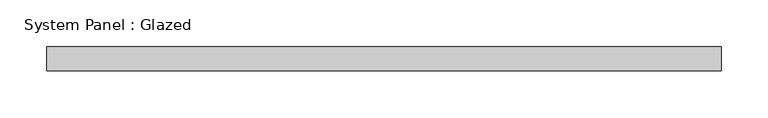
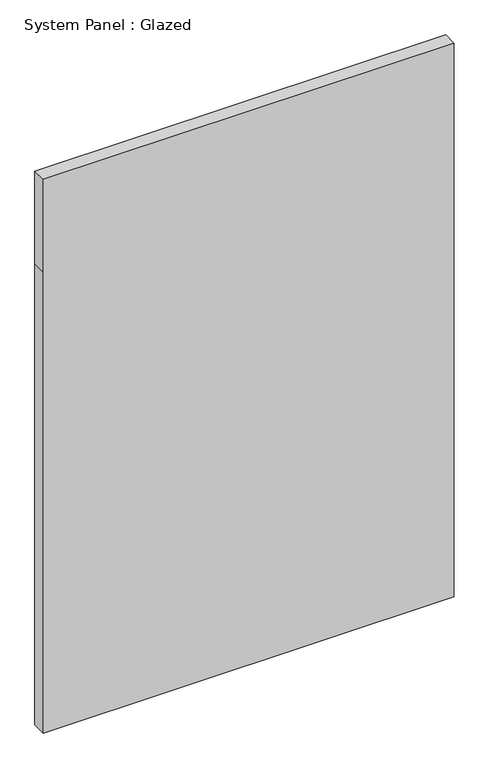
"""IFC4 building model written with IfcOpenShell, lengths in millimetres: plate geometry, System Panel : Glazed."""

from ifc_helpers import new_model, si_unit, frame, origin, place, context, project, spatial, polyline, outline, extrude, source, transform, mapped, element, save


def system_panel_glazed_91241e07(model_context):
    return source(origin(), model_context, "Body", "SweptSolid", [
        extrude(outline(polyline([(0.0, -358.775), (0.0, 358.775), (850.299557, 358.775), (1021.6161252, 358.775), (1021.6161252, -358.775), (850.299557, -358.775), (0.0, -358.775)])), frame((0.0, 19.05, 0.0), z_axis=(0.0, 1.0, 0.0), x_axis=(0.0, 0.0, 1.0)), (0.0, 0.0, 1.0), 25.4),
    ])


if __name__ == "__main__":
    model = new_model("IFC4")
    model_context = context("Model", 3, world=origin())
    ifc_project = project(units=[si_unit("LENGTHUNIT", "METRE", prefix="MILLI")], contexts=[model_context])
    site = spatial("IfcSite", under=ifc_project)
    building = spatial("IfcBuilding", under=site)
    placement = place(None, origin())
    system_panel_glazed_shape = system_panel_glazed_91241e07(model_context)
    element("IfcPlate", 1, ObjectType="System Panel : Glazed", at=placement, inside=building, context=model_context, shape_type="MappedRepresentation", body=[
        mapped(system_panel_glazed_shape, transform((0.0, 0.0, 0.0), x_axis=(1.0, 0.0, 0.0), y_axis=(0.0, 1.0, 0.0), z_axis=(0.0, 0.0, 1.0))),
    ])
    save(model, "model.ifc")

# Revit data of these elements
# Type "System Panel : Glazed"
#   Construction Type Id = "GSP4R"
#   Analytic Construction = "1/8 in Pilkington single glazing"
#   Visual Light Transmittance = 0.9
#   Solar Heat Gain Coefficient = 0.86
#   Heat Transfer Coefficient (U) = 1.18115 BTU/(h·ft²·°F)
#   Define Thermal Properties by = 1
# Element 1 (IfcPlate, "System Panel : Glazed")
#   Materials on its faces: "Glass"
# Materials
#   "Glass": class "Glass", colour RGB 0 128 192, transparency 0.75, Description = "Soda Lime Glass", Cost = 0
